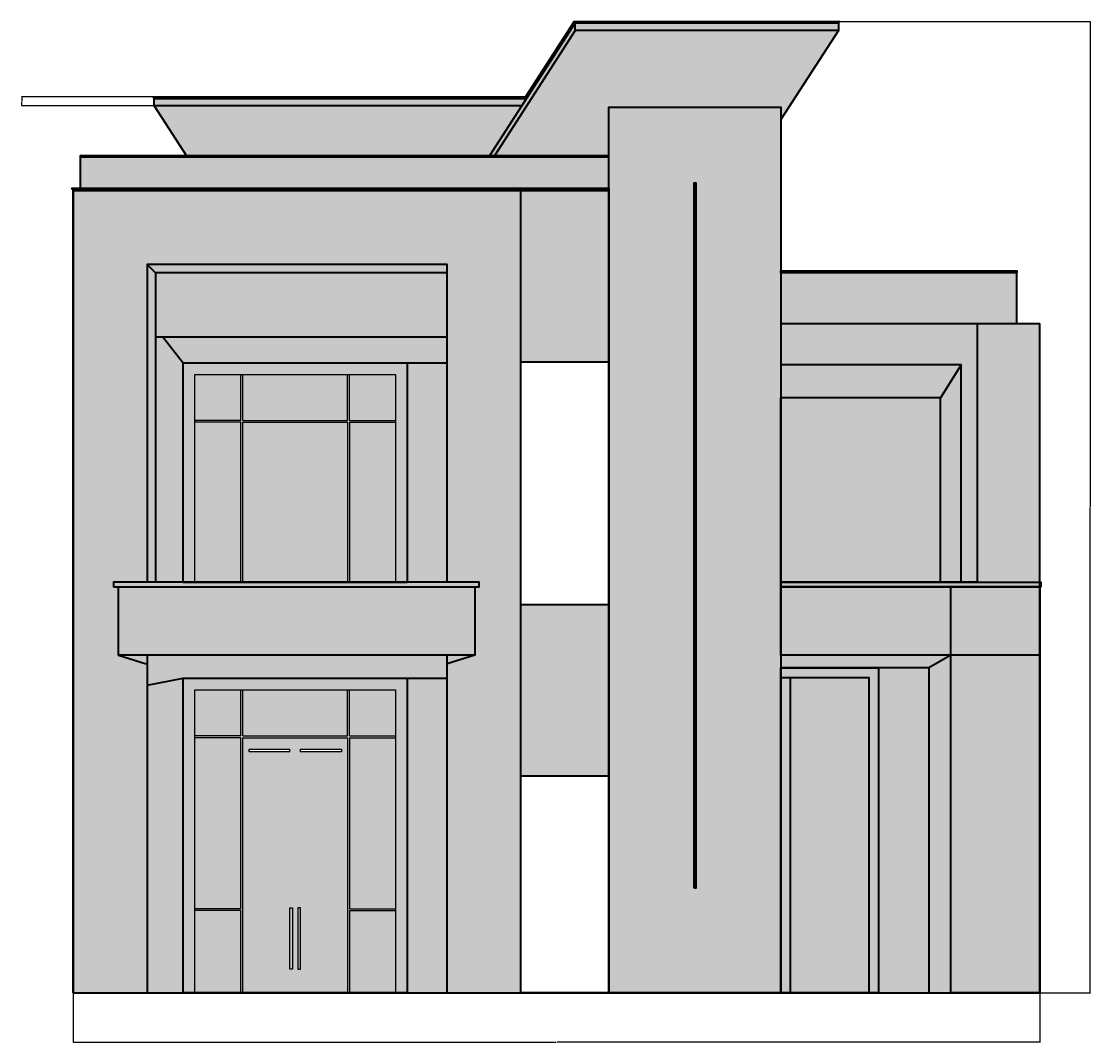
# Model space of a CAD drawing. Units: feet. Extents: x 4092 to 5585, y 725 to 1390.
# Tile 1 of 7: x 4092 to 4756, y 725 to 1359. Entities that reach past the tile are written whole.
import ezdxf

# ---------------------------------------------------------------- set-up
doc = ezdxf.new("R2010")
doc.units = ezdxf.units.FT
for name, color, linetype, lineweight in [('A-ANNO-DIMS', 2, 'Continuous', 18), ('A-DOOR', 3, 'Continuous', 25), ('A-ELEV', 7, 'Continuous', 35), ('A-ELEV-PATT', 8, 'Continuous', 13), ('A-GLAZ', 4, 'Continuous', 25)]:
    doc.layers.add(name, color=color, linetype=linetype, lineweight=lineweight)
doc.styles.get("Standard").update_dxf_attribs({"font": 'arial.ttf'})
doc.dimstyles.get("Standard").update_dxf_attribs({"dimtxt": 0.18, "dimasz": 0.18, "dimexe": 0.18, "dimexo": 0.0625, "dimgap": 0.09, "dimtad": 0, "dimtih": 1, "dimtoh": 1, "dimdec": 1, "dimzin": 0, "dimdsep": 46, "dimlunit": 3, "dimtxsty": 'Standard', "dimcen": 0.09, "dimadec": 0, "dimazin": 0, "dimtfac": 1, "dimtdec": 1, "dimtofl": 0, "dimtmove": 0, "dimatfit": 3, "dimfxl": 1, "dimtolj": 1, "dimtzin": 0, "dimarcsym": 0})

# ---------------------------------------------------------------- blocks, each defined once
blk = doc.blocks.new('*D1')
at = {"layer": 'A-ANNO-DIMS', "color": 0, "lineweight": -2, "transparency": 16777216}
for p, q in [((4124.45, 755.89), (4124.45, 725.07)), ((4724.45, 755.89), (4724.45, 725.07)), ((4124.63, 725.25), (4424.16, 725.25)), ((4724.27, 725.25), (4424.74, 725.25))]:
    blk.add_line(p, q, dxfattribs=at)
at = {"layer": 'A-ANNO-DIMS', "color": 0, "transparency": 16777216}
for points in [[(4124.63, 725.28), (4124.63, 725.22), (4124.45, 725.25)], [(4724.27, 725.28), (4724.27, 725.22), (4724.45, 725.25)]]:
    blk.add_solid(points, dxfattribs=at)
at = {"layer": 'Defpoints', "color": 0, "transparency": 16777216}
for p in [(4124.45, 755.95), (4724.45, 755.95), (4724.45, 725.25)]:
    blk.add_point(p, dxfattribs=at)
at = {"layer": 'A-ANNO-DIMS', "color": 0, "transparency": 16777216, "insert": (4424.45, 725.25), "char_height": 0.18, "attachment_point": 5}
blk.add_mtext('\\A1;600', dxfattribs=at)
blk = doc.blocks.new('*D2')
at = {"layer": 'A-ANNO-DIMS', "color": 0, "lineweight": -2, "transparency": 16777216}
for p, q in [((4435.42, 1358.97), (4755.87, 1358.97)), ((4755.69, 1358.79), (4755.69, 1057.64)), ((4755.69, 756.13), (4755.69, 1057.28)), ((4724.51, 755.95), (4755.87, 755.95))]:
    blk.add_line(p, q, dxfattribs=at)
at = {"layer": 'A-ANNO-DIMS', "color": 0, "transparency": 16777216}
for points in [[(4755.66, 1358.79), (4755.72, 1358.79), (4755.69, 1358.97)], [(4755.66, 756.13), (4755.72, 756.13), (4755.69, 755.95)]]:
    blk.add_solid(points, dxfattribs=at)
at = {"layer": 'Defpoints', "color": 0, "transparency": 16777216}
for p in [(4435.35, 1358.97), (4755.69, 1358.97), (4724.45, 755.95)]:
    blk.add_point(p, dxfattribs=at)
at = {"layer": 'A-ANNO-DIMS', "color": 0, "transparency": 16777216, "insert": (4755.69, 1057.46), "char_height": 0.18, "attachment_point": 5}
blk.add_mtext('\\A1;603', dxfattribs=at)
blk = doc.blocks.new('*D3')
at = {"layer": 'A-ANNO-DIMS', "color": 0, "lineweight": -2, "transparency": 16777216}
for p, q in [((4173.91, 1312.12), (4092.43, 1312.12)), ((4092.61, 1311.94), (4092.61, 1309.49)), ((4092.61, 1306.67), (4092.61, 1309.13)), ((4174.64, 1306.49), (4092.43, 1306.49))]:
    blk.add_line(p, q, dxfattribs=at)
at = {"layer": 'A-ANNO-DIMS', "color": 0, "transparency": 16777216}
for points in [[(4092.58, 1311.94), (4092.64, 1311.94), (4092.61, 1312.12)], [(4092.58, 1306.67), (4092.64, 1306.67), (4092.61, 1306.49)]]:
    blk.add_solid(points, dxfattribs=at)
at = {"layer": 'Defpoints', "color": 0, "transparency": 16777216}
for p in [(4092.61, 1312.12), (4173.97, 1312.12), (4174.71, 1306.49)]:
    blk.add_point(p, dxfattribs=at)
at = {"layer": 'A-ANNO-DIMS', "color": 0, "transparency": 16777216, "insert": (4092.61, 1309.31), "char_height": 0.18, "attachment_point": 5}
blk.add_mtext('\\A1;5.628', dxfattribs=at)

msp = doc.modelspace()

# ---------------------------------------------------------------- hatches: boundary and pattern name
at = {"layer": 'A-ELEV-PATT'}
h = msp.add_hatch(color=256, dxfattribs=at)
h.dxf.hatch_style = 1
h.paths.add_polyline_path([(4170.2715, 1208.1273), (4356.4856, 1208.1273), (4356.4856, 1010.7906), (4376.4327, 1010.7906), (4376.4327, 1007.9488), (4373.6998, 1007.9488), (4373.6998, 965.4789), (4356.4856, 960.128), (4356.4856, 755.9488), (4402.307, 755.9488), (4402.307, 1253.9488), (4124.45, 1253.9488), (4124.45, 755.9488), (4170.2715, 755.9488), (4170.2715, 959.9865), (4152.6018, 965.4789), (4152.6018, 1007.9488), (4149.5131, 1007.9488), (4149.5131, 1010.7906), (4170.2715, 1010.7906)])
h.paths.add_polyline_path([(4373.6998, 1007.9488), (4152.6018, 1007.9488), (4152.6018, 965.4789), (4373.6998, 965.4789)], flags=17)
h.paths.add_polyline_path([(4376.4327, 1010.7906), (4356.4856, 1010.7906), (4149.5131, 1010.7906), (4149.5131, 1007.9488), (4152.6018, 1007.9488), (4376.4327, 1007.9488)], flags=17)
h.paths.add_polyline_path([(4170.2715, 965.4789), (4152.6018, 965.4789), (4170.2715, 959.9865)], flags=17)
h.paths.add_polyline_path([(4373.6998, 965.4789), (4356.4856, 965.4789), (4356.4856, 960.128)], flags=17)
h.paths.add_polyline_path([(4175.4741, 1202.9247), (4170.2715, 1208.1273), (4170.2715, 1010.7906), (4175.4741, 1010.7906)], flags=17)
h.paths.add_polyline_path([(4356.4856, 1208.1273), (4170.2715, 1208.1273), (4175.4741, 1202.9247), (4356.4856, 1202.9247)], flags=17)
h.paths.add_polyline_path([(4563.7091, 1305.7746), (4456.9486, 1305.7746), (4456.9486, 755.9488), (4563.7091, 755.9488)])
h.paths.add_polyline_path([(4510.9094, 820.9207), (4509.7483, 820.9207), (4509.7483, 1258.8497), (4510.9094, 1258.8497)], flags=16)
h.paths.add_polyline_path([(4724.45, 965.4789), (4669.0851, 965.4789), (4669.0851, 755.9488), (4724.45, 755.9488)])
h.paths.add_polyline_path([(4669.0851, 1007.9488), (4563.7091, 1007.9488), (4563.7091, 965.4789), (4669.0851, 965.4789)])
h.paths.add_polyline_path([(4724.45, 1171.511), (4685.4874, 1171.511), (4685.4874, 1010.7906), (4724.45, 1010.7906)])
h.paths.add_polyline_path([(4685.4874, 1171.511), (4563.7091, 1171.511), (4563.7091, 1145.8611), (4675.6205, 1145.8611), (4675.6205, 1010.7906), (4685.4874, 1010.7906)])
h.paths.add_polyline_path([(4599.4061, 1357.9844), (4436.0877, 1357.9844), (4436.0877, 1353.2259), (4599.4061, 1353.2259)])
h.paths.add_polyline_path([(4436.0877, 1353.2259), (4436.0877, 1357.9844), (4382.8181, 1275.5883), (4385.8945, 1275.5883)])
h.paths.add_polyline_path([(4405.7985, 1311.1338), (4174.7061, 1311.1338), (4174.7061, 1306.4942), (4402.799, 1306.4942)])
h = msp.add_hatch(color=256, dxfattribs=at)
h.dxf.hatch_style = 1
h.paths.add_polyline_path([(4599.4061, 1353.2259), (4436.0877, 1353.2259), (4385.8945, 1275.5883), (4456.9486, 1275.5883), (4456.9486, 1305.7746), (4563.7091, 1305.7746), (4563.7091, 1298.0107)])
h.paths.add_polyline_path([(4402.799, 1306.4942), (4174.7061, 1306.4942), (4194.687, 1275.5883), (4382.8181, 1275.5883)])
h.paths.add_polyline_path([(4600.2698, 1358.9731), (4435.3549, 1358.9731), (4436.0877, 1357.9844), (4599.4061, 1357.9844)])
h.paths.add_polyline_path([(4436.0877, 1357.9844), (4435.3549, 1358.9731), (4405.0657, 1312.1225), (4406.4377, 1312.1225)])
h.paths.add_polyline_path([(4406.4377, 1312.1225), (4173.9733, 1312.1225), (4174.7061, 1311.1338), (4405.7985, 1311.1338)])
h.paths.add_polyline_path([(4294.7346, 914.2471), (4229.7185, 914.2471), (4229.7185, 755.9488), (4294.7346, 755.9488)])
h.paths.add_polyline_path([(4233.739, 905.4904), (4233.739, 907.159), (4258.9027, 907.159), (4258.9027, 905.4904)], flags=16)
h.paths.add_polyline_path([(4265.3765, 905.4904), (4265.3765, 907.159), (4290.9761, 907.159), (4290.9761, 905.4904)], flags=16)
h.paths.add_polyline_path([(4258.9959, 808.6527), (4260.6112, 808.6527), (4260.6112, 770.6797), (4258.9959, 770.6797)], flags=16)
h.paths.add_polyline_path([(4263.8419, 808.6527), (4265.4572, 808.6527), (4265.4572, 770.6797), (4263.8419, 770.6797)], flags=16)
h = msp.add_hatch(color=256, dxfattribs=at)
h.dxf.hatch_style = 1
h.paths.add_polyline_path([(4563.7091, 1305.7746), (4456.9486, 1305.7746), (4456.9486, 755.9488), (4563.7091, 755.9488)])
h.paths.add_polyline_path([(4510.9094, 820.9207), (4509.7483, 820.9207), (4509.7483, 1258.8497), (4510.9094, 1258.8497)], flags=16)
h = msp.add_hatch(color=256, dxfattribs=at)
h.dxf.hatch_style = 1
h.paths.add_polyline_path([(4456.9486, 1275.5883), (4128.7842, 1275.5883), (4128.7842, 1274.9372), (4456.9486, 1274.9372)])
h.paths.add_polyline_path([(4510.9094, 1258.8497), (4509.7483, 1258.8497), (4509.7483, 820.9207), (4510.9094, 820.9207)])
h.paths.add_polyline_path([(4624.2143, 957.6463), (4563.7091, 957.6463), (4563.7091, 951.6463), (4569.4033, 951.6463), (4618.2143, 951.6463), (4618.2143, 755.9488), (4624.2143, 755.9488)])
h.paths.add_polyline_path([(4569.4033, 951.6463), (4563.7091, 951.6463), (4563.7091, 755.9488), (4569.4033, 755.9488)], flags=17)
h.paths.add_polyline_path([(4229.7185, 914.2471), (4294.7346, 914.2471), (4294.7346, 755.9488), (4295.9054, 755.9488), (4295.9054, 807.0434), (4324.4959, 807.0434), (4324.4959, 808.2143), (4295.9054, 808.2143), (4295.9054, 914.2471), (4324.4959, 914.2471), (4324.4959, 915.418), (4295.9054, 915.418), (4295.9054, 944.0084), (4294.7346, 944.0084), (4294.7346, 915.418), (4229.7185, 915.418), (4229.7185, 944.0084), (4228.5477, 944.0084), (4228.5477, 915.418), (4199.9573, 915.418), (4199.9573, 914.2471), (4228.5477, 914.2471), (4228.5477, 808.2143), (4199.9573, 808.2143), (4199.9573, 807.0434), (4228.5477, 807.0434), (4228.5477, 755.9488), (4229.7185, 755.9488)])
h.paths.add_polyline_path([(4229.7185, 1110.119), (4294.7346, 1110.119), (4294.7346, 1010.7906), (4295.9054, 1010.7906), (4295.9054, 1110.119), (4324.4959, 1110.119), (4324.4959, 1111.2899), (4295.9054, 1111.2899), (4295.9054, 1139.8803), (4294.7346, 1139.8803), (4294.7346, 1111.2899), (4229.7185, 1111.2899), (4229.7185, 1139.8803), (4228.5477, 1139.8803), (4228.5477, 1111.2899), (4199.9573, 1111.2899), (4199.9573, 1110.119), (4228.5477, 1110.119), (4228.5477, 1010.7906), (4229.7185, 1010.7906)])
h = msp.add_hatch(color=256, dxfattribs=at)
h.dxf.hatch_style = 1
h.paths.add_polyline_path([(4456.9486, 1274.9372), (4128.7842, 1274.9372), (4128.7842, 1255.3673), (4456.9486, 1255.3673)])
h.paths.add_polyline_path([(4228.5477, 1139.8803), (4199.9573, 1139.8803), (4199.9573, 1111.2899), (4228.5477, 1111.2899)])
h.paths.add_polyline_path([(4228.5477, 1110.119), (4199.9573, 1110.119), (4199.9573, 1010.7906), (4228.5477, 1010.7906)])
h.paths.add_polyline_path([(4294.7346, 1139.8803), (4229.7185, 1139.8803), (4229.7185, 1111.2899), (4294.7346, 1111.2899)])
h.paths.add_polyline_path([(4294.7346, 1110.119), (4229.7185, 1110.119), (4229.7185, 1010.7906), (4294.7346, 1010.7906)])
h.paths.add_polyline_path([(4324.4959, 1139.8803), (4295.9054, 1139.8803), (4295.9054, 1111.2899), (4324.4959, 1111.2899)])
h.paths.add_polyline_path([(4324.4959, 1110.119), (4295.9054, 1110.119), (4295.9054, 1010.7906), (4324.4959, 1010.7906)])
h.paths.add_polyline_path([(4228.5477, 944.0084), (4199.9573, 944.0084), (4199.9573, 915.418), (4228.5477, 915.418)])
h.paths.add_polyline_path([(4294.7346, 944.0084), (4229.7185, 944.0084), (4229.7185, 915.418), (4294.7346, 915.418)])
h.paths.add_polyline_path([(4324.4959, 944.0084), (4295.9054, 944.0084), (4295.9054, 915.418), (4324.4959, 915.418)])
h.paths.add_polyline_path([(4324.4959, 914.2471), (4295.9054, 914.2471), (4295.9054, 808.2143), (4324.4959, 808.2143)])
h.paths.add_polyline_path([(4228.5477, 914.2471), (4199.9573, 914.2471), (4199.9573, 808.2143), (4228.5477, 808.2143)])
h.paths.add_polyline_path([(4228.5477, 807.0434), (4199.9573, 807.0434), (4199.9573, 755.9488), (4228.5477, 755.9488)])
h.paths.add_polyline_path([(4324.4959, 807.0434), (4295.9054, 807.0434), (4295.9054, 755.9488), (4324.4959, 755.9488)])
h.paths.add_polyline_path([(4655.4759, 957.6463), (4624.2143, 957.6463), (4624.2143, 755.9488), (4655.4759, 755.9488)])
h.paths.add_polyline_path([(4618.2143, 951.6463), (4569.4033, 951.6463), (4569.4033, 755.9488), (4618.2143, 755.9488)])
h.paths.add_polyline_path([(4662.6345, 1125.3426), (4563.7091, 1125.3426), (4563.7091, 1010.7906), (4662.6345, 1010.7906)])
h = msp.add_hatch(color=256, dxfattribs=at)
h.dxf.hatch_style = 1
h.paths.add_polyline_path([(4356.4856, 1202.9247), (4175.4741, 1202.9247), (4175.4741, 1163.131), (4356.4856, 1163.131)])
h.paths.add_polyline_path([(4331.6899, 1147.0743), (4192.7632, 1147.0743), (4192.7632, 1010.7906), (4199.9573, 1010.7906), (4199.9573, 1139.8803), (4324.4959, 1139.8803), (4324.4959, 1010.7906), (4331.6899, 1010.7906)])
h.paths.add_polyline_path([(4331.6899, 951.2024), (4192.7632, 951.2024), (4192.7632, 755.9488), (4199.9573, 755.9488), (4199.9573, 944.0084), (4324.4959, 944.0084), (4324.4959, 755.9488), (4331.6899, 755.9488)])
h.paths.add_polyline_path([(4724.45, 1010.7906), (4563.7091, 1010.7906), (4563.7091, 1007.9488), (4724.45, 1007.9488)])
h.paths.add_polyline_path([(4724.9893, 1010.7906), (4724.45, 1010.7906), (4724.45, 1007.9488), (4724.9893, 1007.9488)])
h.paths.add_polyline_path([(4456.9486, 1255.3673), (4128.7842, 1255.3673), (4123.3087, 1255.3673), (4124.45, 1253.9488), (4456.9486, 1253.9488)])
h = msp.add_hatch(color=256, dxfattribs=at)
h.dxf.hatch_style = 1
h.paths.add_polyline_path([(4456.9486, 1253.9488), (4402.307, 1253.9488), (4402.307, 1147.5159), (4456.9486, 1147.5159)])
h.paths.add_polyline_path([(4456.9486, 996.9712), (4402.307, 996.9712), (4402.307, 890.5384), (4456.9486, 890.5384)])
h = msp.add_hatch(color=256, dxfattribs=at)
h.dxf.hatch_style = 1
h.paths.add_polyline_path([(4710.0403, 1204.2113), (4563.7091, 1204.2113), (4563.7091, 1202.8338), (4710.0403, 1202.8338)])
h = msp.add_hatch(color=256, dxfattribs=at)
h.dxf.hatch_style = 1
h.paths.add_polyline_path([(4710.0403, 1202.8338), (4563.7091, 1202.8338), (4563.7091, 1171.511), (4710.0403, 1171.511)])
h = msp.add_hatch(color=256, dxfattribs=at)
h.dxf.hatch_style = 1
h.paths.add_polyline_path([(4675.6205, 1145.8611), (4563.7091, 1145.8611), (4563.7091, 1125.3426), (4662.6345, 1125.3426)])
h.paths.add_polyline_path([(4675.6205, 1145.8611), (4662.6345, 1125.3426), (4662.6345, 1010.7906), (4675.6205, 1010.7906)])
h.paths.add_polyline_path([(4192.7632, 1147.0743), (4179.9985, 1163.131), (4175.4741, 1163.131), (4175.4741, 1010.7906), (4192.7632, 1010.7906)])
h.paths.add_polyline_path([(4356.4856, 1163.131), (4179.9985, 1163.131), (4192.7632, 1147.0743), (4331.6899, 1147.0743), (4356.4856, 1147.0743)])
h.paths.add_polyline_path([(4356.4856, 1147.0743), (4331.6899, 1147.0743), (4331.6899, 1010.7906), (4356.4856, 1010.7906)])
h.paths.add_polyline_path([(4192.7632, 951.2024), (4170.2715, 946.8601), (4170.2715, 755.9488), (4192.7632, 755.9488)])
h.paths.add_polyline_path([(4356.4856, 965.4789), (4170.2715, 965.4789), (4170.2715, 946.8601), (4192.7632, 951.2024), (4331.6899, 951.2024), (4356.4856, 951.2024)])
h.paths.add_polyline_path([(4356.4856, 951.2024), (4331.6899, 951.2024), (4331.6899, 755.9488), (4356.4856, 755.9488)])
h.paths.add_polyline_path([(4669.0851, 965.4789), (4655.4759, 957.6463), (4655.4759, 755.9488), (4669.0851, 755.9488)])
h.paths.add_polyline_path([(4669.0851, 965.4789), (4563.7091, 965.4789), (4563.7091, 957.6463), (4624.2143, 957.6463), (4655.4759, 957.6463)])
h = msp.add_hatch(color=256, dxfattribs=at)
h.dxf.hatch_style = 1
h.paths.add_polyline_path([(4724.45, 1007.9488), (4669.0851, 1007.9488), (4669.0851, 965.4789), (4724.45, 965.4789)])
h = msp.add_hatch(color=256, dxfattribs=at)
h.dxf.hatch_style = 1
h.paths.add_polyline_path([(4260.6112, 808.6527), (4258.9959, 808.6527), (4258.9959, 770.6797), (4260.6112, 770.6797)])
h.paths.add_polyline_path([(4265.4572, 808.6527), (4263.8419, 808.6527), (4263.8419, 770.6797), (4265.4572, 770.6797)])

# ---------------------------------------------------------------- linework, layer by layer
at = {"layer": 'A-DOOR'}
for p, q in [((4228.5477, 915.418), (4228.5477, 944.0084)), ((4228.5477, 915.418), (4228.5477, 944.0084)), ((4229.7185, 915.418), (4229.7185, 944.0084)), ((4229.7185, 915.418), (4229.7185, 944.0084)), ((4294.7346, 915.418), (4294.7346, 944.0084)), ((4294.7346, 915.418), (4294.7346, 944.0084)), ((4295.9054, 915.418), (4295.9054, 944.0084)), ((4295.9054, 915.418), (4295.9054, 944.0084)), ((4228.5477, 915.418), (4199.9573, 915.418)), ((4228.5477, 915.418), (4199.9573, 915.418)), ((4228.5477, 914.2471), (4199.9573, 914.2471)), ((4228.5477, 914.2471), (4199.9573, 914.2471)), ((4295.9054, 915.418), (4324.4959, 915.418)), ((4295.9054, 915.418), (4324.4959, 915.418)), ((4295.9054, 914.2471), (4324.4959, 914.2471)), ((4295.9054, 914.2471), (4324.4959, 914.2471)), ((4228.5477, 808.2143), (4199.9573, 808.2143)), ((4228.5477, 808.2143), (4199.9573, 808.2143)), ((4228.5477, 807.0434), (4199.9573, 807.0434)), ((4228.5477, 807.0434), (4199.9573, 807.0434)), ((4295.9054, 808.2143), (4324.4959, 808.2143)), ((4295.9054, 808.2143), (4324.4959, 808.2143)), ((4295.9054, 807.0434), (4324.4959, 807.0434)), ((4295.9054, 807.0434), (4324.4959, 807.0434))]:
    msp.add_line(p, q, dxfattribs=at)
for points in [[(4199.9573, 755.9488), (4199.9573, 944.0084), (4324.4959, 944.0084), (4324.4959, 755.9488)], [(4199.9573, 755.9488), (4199.9573, 944.0084), (4324.4959, 944.0084), (4324.4959, 755.9488)], [(4228.5477, 808.2143), (4228.5477, 914.2471)], [(4228.5477, 808.2143), (4228.5477, 914.2471)], [(4229.7185, 915.418), (4294.7346, 915.418)], [(4229.7185, 915.418), (4294.7346, 915.418)], [(4229.7185, 755.9488), (4229.7185, 914.2471), (4294.7346, 914.2471), (4294.7346, 755.9488)], [(4229.7185, 755.9488), (4229.7185, 914.2471), (4294.7346, 914.2471), (4294.7346, 755.9488)], [(4295.9054, 914.2471), (4295.9054, 808.2143)], [(4295.9054, 914.2471), (4295.9054, 808.2143)], [(4258.9027, 905.4904), (4233.739, 905.4904), (4233.739, 907.159), (4258.9027, 907.159)], [(4258.9027, 905.4904), (4233.739, 905.4904), (4233.739, 907.159), (4258.9027, 907.159)], [(4258.9027, 905.4904), (4258.9027, 907.159)], [(4258.9027, 905.4904), (4258.9027, 907.159)], [(4265.3765, 907.159), (4290.9761, 907.159), (4290.9761, 905.4904), (4265.3765, 905.4904)], [(4265.3765, 907.159), (4265.3765, 905.4904)], [(4265.3765, 907.159), (4290.9761, 907.159), (4290.9761, 905.4904), (4265.3765, 905.4904)], [(4265.3765, 907.159), (4265.3765, 905.4904)], [(4228.5477, 755.9488), (4228.5477, 807.0434)], [(4228.5477, 755.9488), (4228.5477, 807.0434)], [(4295.9054, 807.0434), (4295.9054, 755.9488)], [(4295.9054, 807.0434), (4295.9054, 755.9488)]]:
    msp.add_lwpolyline(points, dxfattribs=at)
for points in [[(4258.9959, 808.6527), (4260.6112, 808.6527), (4260.6112, 770.6797), (4258.9959, 770.6797)], [(4258.9959, 808.6527), (4260.6112, 808.6527), (4260.6112, 770.6797), (4258.9959, 770.6797)], [(4265.4572, 808.6527), (4263.8419, 808.6527), (4263.8419, 770.6797), (4265.4572, 770.6797)], [(4265.4572, 808.6527), (4263.8419, 808.6527), (4263.8419, 770.6797), (4265.4572, 770.6797)]]:
    msp.add_lwpolyline(points, close=True, dxfattribs=at)
at = {"layer": 'A-ELEV'}
for p, q in [((4436.0877, 1357.9844), (4382.8181, 1275.5883)), ((4436.0877, 1357.9844), (4382.8181, 1275.5883)), ((4435.3549, 1358.9731), (4405.0657, 1312.1225)), ((4435.3549, 1358.9731), (4405.0657, 1312.1225)), ((4436.0877, 1353.2259), (4436.0877, 1357.9844)), ((4436.0877, 1353.2259), (4436.0877, 1357.9844)), ((4599.4061, 1357.9844), (4600.2698, 1358.9731)), ((4599.4061, 1357.9844), (4600.2698, 1358.9731)), ((4436.0877, 1353.2259), (4385.8945, 1275.5883)), ((4436.0877, 1353.2259), (4385.8945, 1275.5883)), ((4599.4061, 1353.2259), (4563.7091, 1298.0107)), ((4599.4061, 1353.2259), (4563.7091, 1298.0107)), ((4174.7061, 1306.4942), (4194.687, 1275.5883)), ((4174.7061, 1306.4942), (4194.687, 1275.5883)), ((4124.45, 1253.9488), (4123.3087, 1255.3673)), ((4124.45, 1253.9488), (4123.3087, 1255.3673)), ((4124.45, 755.9488), (4124.45, 1253.9488)), ((4124.45, 1253.9488), (4456.9486, 1253.9488)), ((4124.45, 755.9488), (4124.45, 1253.9488)), ((4124.45, 1253.9488), (4456.9486, 1253.9488)), ((4170.2715, 1208.1273), (4175.4741, 1202.9247)), ((4170.2715, 1208.1273), (4175.4741, 1202.9247)), ((4563.7091, 1171.511), (4724.45, 1171.511)), ((4563.7091, 1171.511), (4724.45, 1171.511)), ((4724.45, 755.9488), (4724.45, 1171.511)), ((4724.45, 755.9488), (4724.45, 1171.511)), ((4175.4741, 1163.131), (4356.4856, 1163.131)), ((4175.4741, 1163.131), (4356.4856, 1163.131)), ((4179.9985, 1163.131), (4192.7632, 1147.0743)), ((4179.9985, 1163.131), (4192.7632, 1147.0743)), ((4331.6899, 1147.0743), (4356.4856, 1147.0743)), ((4331.6899, 1147.0743), (4356.4856, 1147.0743)), ((4675.6205, 1145.8611), (4662.6345, 1125.3426)), ((4675.6205, 1145.8611), (4662.6345, 1125.3426)), ((4192.7632, 1010.7906), (4331.6899, 1010.7906)), ((4192.7632, 1010.7906), (4331.6899, 1010.7906)), ((4152.6018, 965.4789), (4169.8161, 960.128)), ((4152.6018, 965.4789), (4169.8161, 960.128)), ((4373.6998, 965.4789), (4356.4856, 960.128)), ((4373.6998, 965.4789), (4356.4856, 960.128)), ((4669.0851, 965.4789), (4655.4759, 957.6463)), ((4669.0851, 965.4789), (4655.4759, 957.6463)), ((4655.4759, 957.6463), (4563.7091, 957.6463)), ((4655.4759, 957.6463), (4563.7091, 957.6463)), ((4655.4759, 957.6463), (4655.4759, 755.9488)), ((4655.4759, 957.6463), (4655.4759, 755.9488)), ((4170.2715, 946.8601), (4192.7632, 951.2024)), ((4170.2715, 946.8601), (4192.7632, 951.2024)), ((4192.7632, 951.2024), (4356.4856, 951.2024)), ((4192.7632, 951.2024), (4356.4856, 951.2024)), ((4124.45, 755.9488), (4724.45, 755.9488)), ((4124.45, 755.9488), (4724.45, 755.9488))]:
    msp.add_line(p, q, dxfattribs=at)
for points in [[(4599.4061, 1357.9844), (4436.0877, 1357.9844), (4435.3549, 1358.9731), (4600.2698, 1358.9731)], [(4599.4061, 1357.9844), (4436.0877, 1357.9844), (4435.3549, 1358.9731), (4600.2698, 1358.9731)], [(4436.0877, 1357.9844), (4599.4061, 1357.9844), (4599.4061, 1353.2259), (4436.0877, 1353.2259)], [(4436.0877, 1357.9844), (4599.4061, 1357.9844), (4599.4061, 1353.2259), (4436.0877, 1353.2259)], [(4405.7985, 1311.1338), (4174.7061, 1311.1338), (4173.9733, 1312.1225), (4406.4377, 1312.1225)], [(4405.7985, 1311.1338), (4174.7061, 1311.1338), (4173.9733, 1312.1225), (4406.4377, 1312.1225)], [(4402.799, 1306.4942), (4174.7061, 1306.4942), (4174.7061, 1311.1338), (4405.7985, 1311.1338)], [(4402.799, 1306.4942), (4174.7061, 1306.4942), (4174.7061, 1311.1338), (4405.7985, 1311.1338)], [(4123.3087, 1255.3673), (4456.9486, 1255.3673), (4456.9486, 1253.9488), (4124.45, 1253.9488)], [(4123.3087, 1255.3673), (4456.9486, 1255.3673), (4456.9486, 1253.9488), (4124.45, 1253.9488)], [(4356.4856, 1010.7906), (4356.4856, 1208.1273), (4170.2715, 1208.1273), (4170.2715, 1010.7906)], [(4356.4856, 1010.7906), (4356.4856, 1208.1273), (4170.2715, 1208.1273), (4170.2715, 1010.7906)], [(4356.4856, 1202.9247), (4175.4741, 1202.9247), (4175.4741, 1010.7906)], [(4356.4856, 1202.9247), (4175.4741, 1202.9247), (4175.4741, 1010.7906)], [(4685.4874, 1171.511), (4685.4874, 1010.7906), (4563.7091, 1010.7906), (4563.7091, 1125.3426)], [(4685.4874, 1171.511), (4685.4874, 1010.7906), (4563.7091, 1010.7906), (4563.7091, 1125.3426)], [(4192.7632, 1010.7906), (4192.7632, 1147.0743), (4331.6899, 1147.0743), (4331.6899, 1010.7906)], [(4192.7632, 1010.7906), (4192.7632, 1147.0743), (4331.6899, 1147.0743), (4331.6899, 1010.7906)], [(4662.6345, 1010.7906), (4675.6205, 1010.7906), (4675.6205, 1145.8611), (4563.7091, 1145.8611)], [(4662.6345, 1010.7906), (4675.6205, 1010.7906), (4675.6205, 1145.8611), (4563.7091, 1145.8611)], [(4662.6345, 1010.7906), (4662.6345, 1125.3426), (4563.7091, 1125.3426)], [(4662.6345, 1010.7906), (4662.6345, 1125.3426), (4563.7091, 1125.3426)], [(4669.0851, 965.4789), (4563.7091, 965.4789), (4563.7091, 1007.9488), (4724.45, 1007.9488), (4724.45, 965.4789)], [(4669.0851, 1007.9488), (4724.45, 1007.9488), (4724.45, 755.9488), (4669.0851, 755.9488), (4669.0851, 965.4789)], [(4170.2715, 965.4789), (4170.2715, 755.9488)], [(4170.2715, 965.4789), (4170.2715, 755.9488)], [(4356.4856, 755.9488), (4356.4856, 965.4789)], [(4356.4856, 755.9488), (4356.4856, 965.4789)], [(4563.7091, 951.6463), (4618.2143, 951.6463), (4618.2143, 755.9488)], [(4563.7091, 951.6463), (4618.2143, 951.6463), (4618.2143, 755.9488)]]:
    msp.add_lwpolyline(points, dxfattribs=at)
for points in [[(4563.7091, 755.9488), (4456.9486, 755.9488), (4456.9486, 1305.7746), (4563.7091, 1305.7746)], [(4563.7091, 755.9488), (4456.9486, 755.9488), (4456.9486, 1305.7746), (4563.7091, 1305.7746)], [(4128.7842, 1274.9372), (4456.9486, 1274.9372), (4456.9486, 1275.5883), (4128.7842, 1275.5883)], [(4128.7842, 1274.9372), (4456.9486, 1274.9372), (4456.9486, 1275.5883), (4128.7842, 1275.5883)], [(4128.7842, 1255.3673), (4456.9486, 1255.3673), (4456.9486, 1274.9372), (4128.7842, 1274.9372)], [(4128.7842, 1255.3673), (4456.9486, 1255.3673), (4456.9486, 1274.9372), (4128.7842, 1274.9372)], [(4509.7483, 820.9207), (4509.7483, 1258.8497), (4510.9094, 1258.8497), (4510.9094, 820.9207)], [(4509.7483, 820.9207), (4509.7483, 1258.8497), (4510.9094, 1258.8497), (4510.9094, 820.9207)], [(4124.45, 755.9488), (4402.307, 755.9488), (4402.307, 1253.9488), (4124.45, 1253.9488)], [(4124.45, 755.9488), (4402.307, 755.9488), (4402.307, 1253.9488), (4124.45, 1253.9488)], [(4402.307, 1253.9488), (4456.9486, 1253.9488), (4456.9486, 755.9488), (4402.307, 755.9488)], [(4402.307, 1253.9488), (4456.9486, 1253.9488), (4456.9486, 1147.5159), (4402.307, 1147.5159)], [(4402.307, 1253.9488), (4456.9486, 1253.9488), (4456.9486, 755.9488), (4402.307, 755.9488)], [(4402.307, 1253.9488), (4456.9486, 1253.9488), (4456.9486, 1147.5159), (4402.307, 1147.5159)], [(4710.0403, 1202.8338), (4563.7091, 1202.8338), (4563.7091, 1204.2113), (4710.0403, 1204.2113)], [(4710.0403, 1202.8338), (4563.7091, 1202.8338), (4563.7091, 1204.2113), (4710.0403, 1204.2113)], [(4563.7091, 1171.511), (4710.0403, 1171.511), (4710.0403, 1202.8338), (4563.7091, 1202.8338)], [(4563.7091, 1171.511), (4710.0403, 1171.511), (4710.0403, 1202.8338), (4563.7091, 1202.8338)], [(4149.5131, 1007.9488), (4376.4327, 1007.9488), (4376.4327, 1010.7906), (4149.5131, 1010.7906)], [(4149.5131, 1007.9488), (4376.4327, 1007.9488), (4376.4327, 1010.7906), (4149.5131, 1010.7906)], [(4563.7091, 1010.7906), (4724.9893, 1010.7906), (4724.9893, 1007.9488), (4563.7091, 1007.9488)], [(4563.7091, 1010.7906), (4724.9893, 1010.7906), (4724.9893, 1007.9488), (4563.7091, 1007.9488)], [(4152.6018, 1007.9488), (4373.6998, 1007.9488), (4373.6998, 965.4789), (4152.6018, 965.4789)], [(4152.6018, 1007.9488), (4373.6998, 1007.9488), (4373.6998, 965.4789), (4152.6018, 965.4789)], [(4563.7091, 1007.9488), (4724.45, 1007.9488), (4724.45, 965.4789), (4563.7091, 965.4789)], [(4724.45, 755.9488), (4669.0851, 755.9488), (4669.0851, 1007.9488), (4724.45, 1007.9488)], [(4402.307, 996.9712), (4456.9486, 996.9712), (4456.9486, 890.5384), (4402.307, 890.5384)], [(4402.307, 996.9712), (4456.9486, 996.9712), (4456.9486, 890.5384), (4402.307, 890.5384)], [(4563.7091, 957.6463), (4624.2143, 957.6463), (4624.2143, 755.9488), (4563.7091, 755.9488)], [(4563.7091, 957.6463), (4624.2143, 957.6463), (4624.2143, 755.9488), (4563.7091, 755.9488)], [(4192.7632, 951.2024), (4331.6899, 951.2024), (4331.6899, 755.9488), (4192.7632, 755.9488)], [(4192.7632, 951.2024), (4331.6899, 951.2024), (4331.6899, 755.9488), (4192.7632, 755.9488)], [(4563.7091, 951.6463), (4569.4033, 951.6463), (4569.4033, 755.9488), (4563.7091, 755.9488)], [(4563.7091, 951.6463), (4569.4033, 951.6463), (4569.4033, 755.9488), (4563.7091, 755.9488)]]:
    msp.add_lwpolyline(points, close=True, dxfattribs=at)
at = {"layer": 'A-GLAZ'}
for p, q in [((4228.5477, 1111.2899), (4228.5477, 1139.8803)), ((4228.5477, 1111.2899), (4228.5477, 1139.8803)), ((4229.7185, 1111.2899), (4229.7185, 1139.8803)), ((4229.7185, 1111.2899), (4229.7185, 1139.8803)), ((4294.7346, 1111.2899), (4294.7346, 1139.8803)), ((4294.7346, 1111.2899), (4294.7346, 1139.8803)), ((4295.9054, 1111.2899), (4295.9054, 1139.8803)), ((4295.9054, 1111.2899), (4295.9054, 1139.8803)), ((4228.5477, 1111.2899), (4199.9573, 1111.2899)), ((4228.5477, 1111.2899), (4199.9573, 1111.2899)), ((4228.5477, 1110.119), (4199.9573, 1110.119)), ((4228.5477, 1110.119), (4199.9573, 1110.119)), ((4295.9054, 1111.2899), (4324.4959, 1111.2899)), ((4295.9054, 1111.2899), (4324.4959, 1111.2899)), ((4295.9054, 1110.119), (4324.4959, 1110.119)), ((4295.9054, 1110.119), (4324.4959, 1110.119))]:
    msp.add_line(p, q, dxfattribs=at)
for points in [[(4199.9573, 1010.7906), (4199.9573, 1139.8803), (4324.4959, 1139.8803), (4324.4959, 1010.7906)], [(4199.9573, 1010.7906), (4199.9573, 1139.8803), (4324.4959, 1139.8803), (4324.4959, 1010.7906)], [(4228.5477, 1010.7906), (4228.5477, 1110.119)], [(4228.5477, 1010.7906), (4228.5477, 1110.119)], [(4229.7185, 1111.2899), (4294.7346, 1111.2899)], [(4229.7185, 1111.2899), (4294.7346, 1111.2899)], [(4229.7185, 1010.7906), (4229.7185, 1110.119), (4294.7346, 1110.119), (4294.7346, 1010.7906)], [(4229.7185, 1010.7906), (4229.7185, 1110.119), (4294.7346, 1110.119), (4294.7346, 1010.7906)], [(4295.9054, 1110.119), (4295.9054, 1010.7906)], [(4295.9054, 1110.119), (4295.9054, 1010.7906)]]:
    msp.add_lwpolyline(points, dxfattribs=at)

# ---------------------------------------------------------------- dimensions: what is measured, and where the dimension line sits
at = {"layer": 'A-ANNO-DIMS'}
for base, p1, p2, override, picture, middle in [((4755.6893, 1358.9731), (4724.45, 755.9488), (4435.3549, 1358.9731), {"dimdec": 0, "dimlfac": 1, "dimrnd": 0, "dimzin": 0, "dimdsep": 46, "dimlunit": 2}, '*D2', (4755.6893, 1057.461)), ((4092.6087, 1312.1225), (4174.7061, 1306.4942), (4173.9733, 1312.1225), {"dimdec": 3, "dimlfac": 1, "dimrnd": 0, "dimzin": 0, "dimdsep": 46, "dimlunit": 2}, '*D3', (4092.6087, 1309.3083))]:
    dim = msp.add_linear_dim(base=base, p1=p1, p2=p2, angle=90, dimstyle='Standard', override=override, dxfattribs=at)
    dim.commit()
    dim.dimension.update_dxf_attribs({"geometry": picture, "text_midpoint": middle})
dim = msp.add_linear_dim(base=(4724.45, 725.2488), p1=(4124.45, 755.9488), p2=(4724.45, 755.9488), dimstyle='Standard', override={"dimdec": 0, "dimlfac": 1, "dimrnd": 0, "dimzin": 0, "dimdsep": 46, "dimlunit": 2}, dxfattribs=at)
dim.commit()
dim.dimension.update_dxf_attribs({"geometry": '*D1', "text_midpoint": (4424.45, 725.2488)})

doc.saveas('drawing.dxf')
